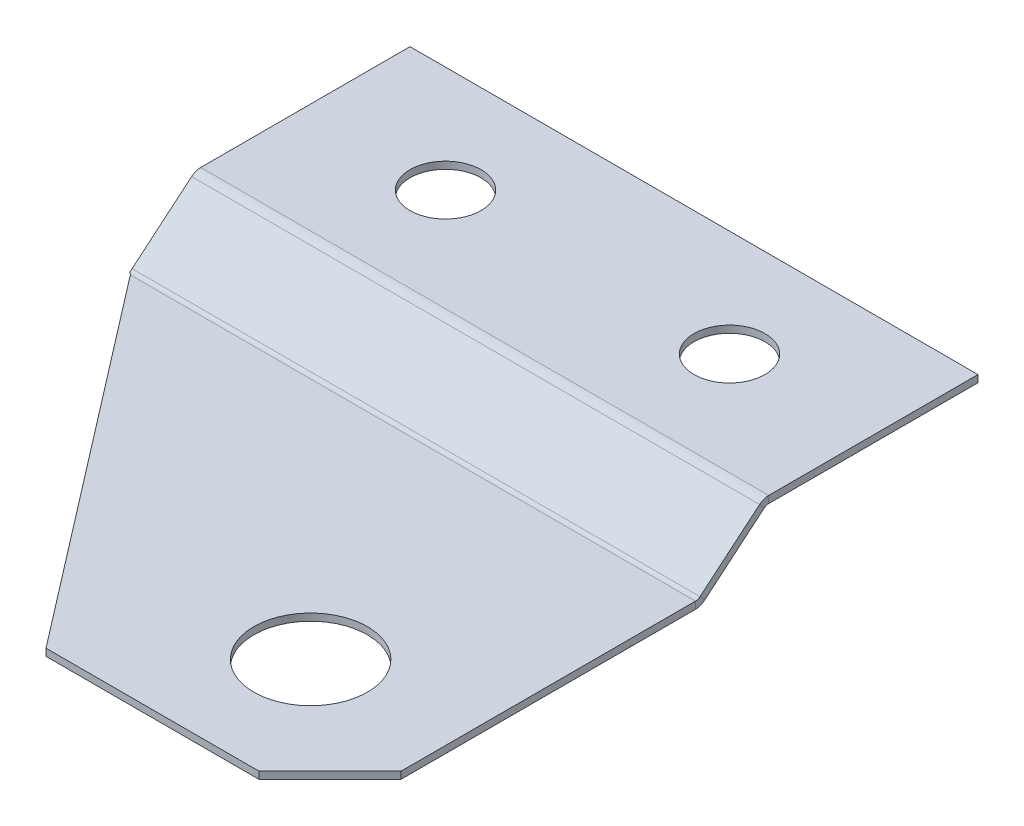
ISO-10303-21;
HEADER;
FILE_DESCRIPTION(('STEP AP214'),'2;1');
FILE_NAME('part.step','',(''),(''),'','','');
FILE_SCHEMA(('AUTOMOTIVE_DESIGN { 1 0 10303 214 1 1 1 1 }'));
ENDSEC;
DATA;
#1=APPLICATION_CONTEXT('core data for automotive mechanical design processes');
#2=APPLICATION_PROTOCOL_DEFINITION('international standard','automotive_design',2000,#1);
#3=PRODUCT_CONTEXT('',#1,'mechanical');
#4=PRODUCT('Part','Part','',(#3));
#5=PRODUCT_RELATED_PRODUCT_CATEGORY('part','',(#4));
#6=PRODUCT_DEFINITION_FORMATION('','',#4);
#7=PRODUCT_DEFINITION_CONTEXT('part definition',#1,'design');
#8=PRODUCT_DEFINITION('design','',#6,#7);
#9=PRODUCT_DEFINITION_SHAPE('','',#8);
#10=(LENGTH_UNIT() NAMED_UNIT(*) SI_UNIT(.MILLI.,.METRE.));
#11=(NAMED_UNIT(*) PLANE_ANGLE_UNIT() SI_UNIT($,.RADIAN.));
#12=(NAMED_UNIT(*) SI_UNIT($,.STERADIAN.) SOLID_ANGLE_UNIT());
#13=UNCERTAINTY_MEASURE_WITH_UNIT(LENGTH_MEASURE(1.E-05),#10,'distance_accuracy_value','');
#14=(GEOMETRIC_REPRESENTATION_CONTEXT(3) GLOBAL_UNCERTAINTY_ASSIGNED_CONTEXT((#13)) GLOBAL_UNIT_ASSIGNED_CONTEXT((#10,
#11,#12)) REPRESENTATION_CONTEXT('',''));
#15=CARTESIAN_POINT('',(0.,0.,0.));
#16=DIRECTION('',(0.,0.,1.));
#17=DIRECTION('',(1.,0.,0.));
#18=AXIS2_PLACEMENT_3D('',#15,#16,#17);
#19=CARTESIAN_POINT('',(0.,2.44384786784973,0.911844456773233));
#20=DIRECTION('',(0.,0.766044443118977,0.642787609686541));
#21=DIRECTION('',(0.,-0.642787609686541,0.766044443118977));
#22=AXIS2_PLACEMENT_3D('',#19,#20,#21);
#23=PLANE('',#22);
#24=DIRECTION('',(0.,0.64278760968654,-0.766044443118977));
#25=VECTOR('',#24,1.);
#26=CARTESIAN_POINT('',(20.,9.19311776955841,-7.13162219597603));
#27=LINE('',#26,#25);
#28=CARTESIAN_POINT('',(20.,-4.13714063115813,8.75476114328701));
#29=VERTEX_POINT('',#28);
#30=CARTESIAN_POINT('',(20.,-0.616977778440511,4.55959441704411));
#31=VERTEX_POINT('',#30);
#32=EDGE_CURVE('E375',#29,#31,#27,.T.);
#33=ORIENTED_EDGE('',*,*,#32,.F.);
#34=DIRECTION('',(-1.,0.,0.));
#35=VECTOR('',#34,1.);
#36=CARTESIAN_POINT('',(0.,-4.13714063115813,8.754761143287));
#37=LINE('',#36,#35);
#38=CARTESIAN_POINT('',(-20.,-4.13714063115813,8.75476114328701));
#39=VERTEX_POINT('',#38);
#40=EDGE_CURVE('E361',#29,#39,#37,.T.);
#41=ORIENTED_EDGE('',*,*,#40,.T.);
#42=DIRECTION('',(0.,-0.64278760968654,0.766044443118977));
#43=VECTOR('',#42,1.);
#44=CARTESIAN_POINT('',(-20.,9.19311776955841,-7.13162219597603));
#45=LINE('',#44,#43);
#46=CARTESIAN_POINT('',(-20.,-0.61697777844051,4.55959441704412));
#47=VERTEX_POINT('',#46);
#48=EDGE_CURVE('E357',#47,#39,#45,.T.);
#49=ORIENTED_EDGE('',*,*,#48,.F.);
#50=DIRECTION('',(-1.,0.,0.));
#51=VECTOR('',#50,1.);
#52=CARTESIAN_POINT('',(0.,-0.616977778440513,4.55959441704412));
#53=LINE('',#52,#51);
#54=EDGE_CURVE('E352',#31,#47,#53,.T.);
#55=ORIENTED_EDGE('',*,*,#54,.F.);
#56=EDGE_LOOP('',(#33,#41,#49,#55));
#57=FACE_BOUND('',#56,.T.);
#58=ADVANCED_FACE('F56',(#57),#23,.F.);
#59=CARTESIAN_POINT('',(20.,9.19311776955841,-7.13162219597603));
#60=DIRECTION('',(1.,0.,0.));
#61=DIRECTION('',(0.,0.642787609686541,-0.766044443118977));
#62=AXIS2_PLACEMENT_3D('',#59,#60,#61);
#63=PLANE('',#62);
#64=DIRECTION('',(0.,0.766044443118977,0.64278760968654));
#65=VECTOR('',#64,1.);
#66=CARTESIAN_POINT('',(20.,-4.13714063115813,8.75476114328701));
#67=LINE('',#66,#65);
#68=CARTESIAN_POINT('',(20.,-3.75411840959864,9.07615494813028));
#69=VERTEX_POINT('',#68);
#70=EDGE_CURVE('E366',#29,#69,#67,.T.);
#71=ORIENTED_EDGE('',*,*,#70,.F.);
#72=ORIENTED_EDGE('',*,*,#32,.T.);
#73=DIRECTION('',(0.,0.766044443118977,0.642787609686541));
#74=VECTOR('',#73,1.);
#75=CARTESIAN_POINT('',(20.,-0.616977778440512,4.55959441704412));
#76=LINE('',#75,#74);
#77=CARTESIAN_POINT('',(20.,-0.233955556881022,4.88098822188738));
#78=VERTEX_POINT('',#77);
#79=EDGE_CURVE('E363',#31,#78,#76,.T.);
#80=ORIENTED_EDGE('',*,*,#79,.T.);
#81=DIRECTION('',(0.,0.64278760968654,-0.766044443118977));
#82=VECTOR('',#81,1.);
#83=CARTESIAN_POINT('',(20.,9.5761399911179,-6.81022839113276));
#84=LINE('',#83,#82);
#85=EDGE_CURVE('E86',#69,#78,#84,.T.);
#86=ORIENTED_EDGE('',*,*,#85,.F.);
#87=EDGE_LOOP('',(#71,#72,#80,#86));
#88=FACE_BOUND('',#87,.T.);
#89=ADVANCED_FACE('F425',(#88),#63,.T.);
#90=CARTESIAN_POINT('',(-20.,9.19311776955841,-7.13162219597603));
#91=DIRECTION('',(-1.,0.,0.));
#92=DIRECTION('',(0.,-0.642787609686541,0.766044443118977));
#93=AXIS2_PLACEMENT_3D('',#90,#91,#92);
#94=PLANE('',#93);
#95=DIRECTION('',(0.,-0.766044443118977,-0.64278760968654));
#96=VECTOR('',#95,1.);
#97=CARTESIAN_POINT('',(-20.,-4.13714063115812,8.754761143287));
#98=LINE('',#97,#96);
#99=CARTESIAN_POINT('',(-20.,-3.75411840959864,9.07615494813028));
#100=VERTEX_POINT('',#99);
#101=EDGE_CURVE('E12',#100,#39,#98,.T.);
#102=ORIENTED_EDGE('',*,*,#101,.F.);
#103=DIRECTION('',(0.,-0.64278760968654,0.766044443118977));
#104=VECTOR('',#103,1.);
#105=CARTESIAN_POINT('',(-20.,9.5761399911179,-6.81022839113276));
#106=LINE('',#105,#104);
#107=CARTESIAN_POINT('',(-20.,-0.233955556881022,4.88098822188738));
#108=VERTEX_POINT('',#107);
#109=EDGE_CURVE('E76',#108,#100,#106,.T.);
#110=ORIENTED_EDGE('',*,*,#109,.F.);
#111=DIRECTION('',(0.,-0.766044443118977,-0.642787609686541));
#112=VECTOR('',#111,1.);
#113=CARTESIAN_POINT('',(-20.,-0.616977778440512,4.55959441704412));
#114=LINE('',#113,#112);
#115=EDGE_CURVE('E358',#108,#47,#114,.T.);
#116=ORIENTED_EDGE('',*,*,#115,.T.);
#117=ORIENTED_EDGE('',*,*,#48,.T.);
#118=EDGE_LOOP('',(#102,#110,#116,#117));
#119=FACE_BOUND('',#118,.T.);
#120=ADVANCED_FACE('F431',(#119),#94,.T.);
#121=CARTESIAN_POINT('',(0.,2.82687008940922,1.2332382616165));
#122=DIRECTION('',(0.,0.766044443118977,0.642787609686541));
#123=DIRECTION('',(0.,-0.642787609686541,0.766044443118977));
#124=AXIS2_PLACEMENT_3D('',#121,#122,#123);
#125=PLANE('',#124);
#126=DIRECTION('',(-1.,0.,0.));
#127=VECTOR('',#126,1.);
#128=CARTESIAN_POINT('',(0.,-3.75411840959864,9.07615494813028));
#129=LINE('',#128,#127);
#130=EDGE_CURVE('E67',#69,#100,#129,.T.);
#131=ORIENTED_EDGE('',*,*,#130,.F.);
#132=ORIENTED_EDGE('',*,*,#85,.T.);
#133=DIRECTION('',(-1.,0.,0.));
#134=VECTOR('',#133,1.);
#135=CARTESIAN_POINT('',(0.,-0.233955556881024,4.88098822188739));
#136=LINE('',#135,#134);
#137=EDGE_CURVE('E360',#78,#108,#136,.T.);
#138=ORIENTED_EDGE('',*,*,#137,.T.);
#139=ORIENTED_EDGE('',*,*,#109,.T.);
#140=EDGE_LOOP('',(#131,#132,#138,#139));
#141=FACE_BOUND('',#140,.T.);
#142=ADVANCED_FACE('F63',(#141),#125,.T.);
#143=CARTESIAN_POINT('',(-20.,-0.5,-10.5));
#144=DIRECTION('',(0.,0.,-1.));
#145=DIRECTION('',(-1.,0.,0.));
#146=AXIS2_PLACEMENT_3D('',#143,#144,#145);
#147=PLANE('',#146);
#148=DIRECTION('',(-1.,0.,0.));
#149=VECTOR('',#148,1.);
#150=CARTESIAN_POINT('',(-20.,0.,-10.5));
#151=LINE('',#150,#149);
#152=CARTESIAN_POINT('',(20.,0.,-10.5));
#153=VERTEX_POINT('',#152);
#154=CARTESIAN_POINT('',(-20.,0.,-10.5));
#155=VERTEX_POINT('',#154);
#156=EDGE_CURVE('E327',#153,#155,#151,.T.);
#157=ORIENTED_EDGE('',*,*,#156,.F.);
#158=DIRECTION('',(0.,1.,0.));
#159=VECTOR('',#158,1.);
#160=CARTESIAN_POINT('',(20.,-0.5,-10.5));
#161=LINE('',#160,#159);
#162=CARTESIAN_POINT('',(20.,-0.5,-10.5));
#163=VERTEX_POINT('',#162);
#164=EDGE_CURVE('E321',#163,#153,#161,.T.);
#165=ORIENTED_EDGE('',*,*,#164,.F.);
#166=DIRECTION('',(-1.,0.,0.));
#167=VECTOR('',#166,1.);
#168=CARTESIAN_POINT('',(-20.,-0.5,-10.5));
#169=LINE('',#168,#167);
#170=CARTESIAN_POINT('',(-20.,-0.5,-10.5));
#171=VERTEX_POINT('',#170);
#172=EDGE_CURVE('E345',#163,#171,#169,.T.);
#173=ORIENTED_EDGE('',*,*,#172,.T.);
#174=DIRECTION('',(0.,1.,0.));
#175=VECTOR('',#174,1.);
#176=CARTESIAN_POINT('',(-20.,-0.5,-10.5));
#177=LINE('',#176,#175);
#178=EDGE_CURVE('E338',#171,#155,#177,.T.);
#179=ORIENTED_EDGE('',*,*,#178,.T.);
#180=EDGE_LOOP('',(#157,#165,#173,#179));
#181=FACE_BOUND('',#180,.T.);
#182=ADVANCED_FACE('F455',(#181),#147,.T.);
#183=CARTESIAN_POINT('',(0.,-0.5,0.));
#184=DIRECTION('',(0.,1.,0.));
#185=DIRECTION('',(0.,0.,1.));
#186=AXIS2_PLACEMENT_3D('',#183,#184,#185);
#187=PLANE('',#186);
#188=CARTESIAN_POINT('',(-10.,-0.5,-3.));
#189=DIRECTION('',(0.,1.,0.));
#190=DIRECTION('',(0.,0.,1.));
#191=AXIS2_PLACEMENT_3D('',#188,#189,#190);
#192=CIRCLE('',#191,2.5);
#193=CARTESIAN_POINT('',(-10.,-0.5,-0.500000000000002));
#194=VERTEX_POINT('',#193);
#195=EDGE_CURVE('E195',#194,#194,#192,.T.);
#196=ORIENTED_EDGE('',*,*,#195,.T.);
#197=EDGE_LOOP('',(#196));
#198=FACE_BOUND('',#197,.T.);
#199=CARTESIAN_POINT('',(10.,-0.5,-3.));
#200=DIRECTION('',(0.,1.,0.));
#201=DIRECTION('',(0.,0.,1.));
#202=AXIS2_PLACEMENT_3D('',#199,#200,#201);
#203=CIRCLE('',#202,2.5);
#204=CARTESIAN_POINT('',(10.,-0.5,-0.500000000000002));
#205=VERTEX_POINT('',#204);
#206=EDGE_CURVE('E650',#205,#205,#203,.T.);
#207=ORIENTED_EDGE('',*,*,#206,.T.);
#208=EDGE_LOOP('',(#207));
#209=FACE_BOUND('',#208,.T.);
#210=DIRECTION('',(0.,0.,-1.));
#211=VECTOR('',#210,1.);
#212=CARTESIAN_POINT('',(20.,-0.5,-10.5));
#213=LINE('',#212,#211);
#214=CARTESIAN_POINT('',(20.,-0.5,4.23820061220084));
#215=VERTEX_POINT('',#214);
#216=EDGE_CURVE('E329',#215,#163,#213,.T.);
#217=ORIENTED_EDGE('',*,*,#216,.F.);
#218=DIRECTION('',(-1.,0.,0.));
#219=VECTOR('',#218,1.);
#220=CARTESIAN_POINT('',(0.,-0.5,4.23820061220085));
#221=LINE('',#220,#219);
#222=CARTESIAN_POINT('',(-20.,-0.5,4.23820061220084));
#223=VERTEX_POINT('',#222);
#224=EDGE_CURVE('E340',#215,#223,#221,.T.);
#225=ORIENTED_EDGE('',*,*,#224,.T.);
#226=DIRECTION('',(0.,0.,1.));
#227=VECTOR('',#226,1.);
#228=CARTESIAN_POINT('',(-20.,-0.5,-10.5));
#229=LINE('',#228,#227);
#230=EDGE_CURVE('E334',#171,#223,#229,.T.);
#231=ORIENTED_EDGE('',*,*,#230,.F.);
#232=ORIENTED_EDGE('',*,*,#172,.F.);
#233=EDGE_LOOP('',(#217,#225,#231,#232));
#234=FACE_BOUND('',#233,.T.);
#235=ADVANCED_FACE('F449',(#198,#209,#234),#187,.F.);
#236=CARTESIAN_POINT('',(-20.,-0.5,-10.5));
#237=DIRECTION('',(-1.,0.,0.));
#238=DIRECTION('',(0.,0.,1.));
#239=AXIS2_PLACEMENT_3D('',#236,#237,#238);
#240=PLANE('',#239);
#241=DIRECTION('',(0.,-1.,0.));
#242=VECTOR('',#241,1.);
#243=CARTESIAN_POINT('',(-20.,-0.499999999999999,4.23820061220085));
#244=LINE('',#243,#242);
#245=CARTESIAN_POINT('',(-20.,0.,4.23820061220084));
#246=VERTEX_POINT('',#245);
#247=EDGE_CURVE('E342',#246,#223,#244,.T.);
#248=ORIENTED_EDGE('',*,*,#247,.F.);
#249=DIRECTION('',(0.,0.,1.));
#250=VECTOR('',#249,1.);
#251=CARTESIAN_POINT('',(-20.,0.,-10.5));
#252=LINE('',#251,#250);
#253=EDGE_CURVE('E330',#155,#246,#252,.T.);
#254=ORIENTED_EDGE('',*,*,#253,.F.);
#255=ORIENTED_EDGE('',*,*,#178,.F.);
#256=ORIENTED_EDGE('',*,*,#230,.T.);
#257=EDGE_LOOP('',(#248,#254,#255,#256));
#258=FACE_BOUND('',#257,.T.);
#259=ADVANCED_FACE('F443',(#258),#240,.T.);
#260=CARTESIAN_POINT('',(0.,0.,0.));
#261=DIRECTION('',(0.,1.,0.));
#262=DIRECTION('',(0.,0.,1.));
#263=AXIS2_PLACEMENT_3D('',#260,#261,#262);
#264=PLANE('',#263);
#265=CARTESIAN_POINT('',(-10.,0.,-3.));
#266=DIRECTION('',(0.,1.,0.));
#267=DIRECTION('',(0.,0.,1.));
#268=AXIS2_PLACEMENT_3D('',#265,#266,#267);
#269=CIRCLE('',#268,2.5);
#270=CARTESIAN_POINT('',(-10.,0.,-0.500000000000002));
#271=VERTEX_POINT('',#270);
#272=EDGE_CURVE('E651',#271,#271,#269,.T.);
#273=ORIENTED_EDGE('',*,*,#272,.F.);
#274=EDGE_LOOP('',(#273));
#275=FACE_BOUND('',#274,.T.);
#276=CARTESIAN_POINT('',(10.,0.,-3.));
#277=DIRECTION('',(0.,1.,0.));
#278=DIRECTION('',(0.,0.,1.));
#279=AXIS2_PLACEMENT_3D('',#276,#277,#278);
#280=CIRCLE('',#279,2.5);
#281=CARTESIAN_POINT('',(10.,0.,-0.500000000000002));
#282=VERTEX_POINT('',#281);
#283=EDGE_CURVE('E652',#282,#282,#280,.T.);
#284=ORIENTED_EDGE('',*,*,#283,.F.);
#285=EDGE_LOOP('',(#284));
#286=FACE_BOUND('',#285,.T.);
#287=DIRECTION('',(-1.,0.,0.));
#288=VECTOR('',#287,1.);
#289=CARTESIAN_POINT('',(0.,0.,4.23820061220085));
#290=LINE('',#289,#288);
#291=CARTESIAN_POINT('',(20.,0.,4.23820061220084));
#292=VERTEX_POINT('',#291);
#293=EDGE_CURVE('E348',#292,#246,#290,.T.);
#294=ORIENTED_EDGE('',*,*,#293,.F.);
#295=DIRECTION('',(0.,0.,-1.));
#296=VECTOR('',#295,1.);
#297=CARTESIAN_POINT('',(20.,0.,-10.5));
#298=LINE('',#297,#296);
#299=EDGE_CURVE('E333',#292,#153,#298,.T.);
#300=ORIENTED_EDGE('',*,*,#299,.T.);
#301=ORIENTED_EDGE('',*,*,#156,.T.);
#302=ORIENTED_EDGE('',*,*,#253,.T.);
#303=EDGE_LOOP('',(#294,#300,#301,#302));
#304=FACE_BOUND('',#303,.T.);
#305=ADVANCED_FACE('F439',(#275,#286,#304),#264,.T.);
#306=CARTESIAN_POINT('',(20.,-0.5,-10.5));
#307=DIRECTION('',(1.,0.,0.));
#308=DIRECTION('',(0.,0.,-1.));
#309=AXIS2_PLACEMENT_3D('',#306,#307,#308);
#310=PLANE('',#309);
#311=DIRECTION('',(0.,1.,0.));
#312=VECTOR('',#311,1.);
#313=CARTESIAN_POINT('',(20.,-0.499999999999999,4.23820061220085));
#314=LINE('',#313,#312);
#315=EDGE_CURVE('E320',#215,#292,#314,.T.);
#316=ORIENTED_EDGE('',*,*,#315,.F.);
#317=ORIENTED_EDGE('',*,*,#216,.T.);
#318=ORIENTED_EDGE('',*,*,#164,.T.);
#319=ORIENTED_EDGE('',*,*,#299,.F.);
#320=EDGE_LOOP('',(#316,#317,#318,#319));
#321=FACE_BOUND('',#320,.T.);
#322=ADVANCED_FACE('F436',(#321),#310,.T.);
#323=CARTESIAN_POINT('',(20.,-1.,4.23820061220085));
#324=DIRECTION('',(-1.,0.,0.));
#325=DIRECTION('',(0.,0.,1.));
#326=AXIS2_PLACEMENT_3D('',#323,#324,#325);
#327=PLANE('',#326);
#328=ORIENTED_EDGE('',*,*,#315,.T.);
#329=CARTESIAN_POINT('',(20.,-1.,4.23820061220085));
#330=DIRECTION('',(-1.,0.,0.));
#331=DIRECTION('',(0.,0.,1.));
#332=AXIS2_PLACEMENT_3D('',#329,#330,#331);
#333=CIRCLE('',#332,1.);
#334=EDGE_CURVE('E318',#292,#78,#333,.F.);
#335=ORIENTED_EDGE('',*,*,#334,.T.);
#336=ORIENTED_EDGE('',*,*,#79,.F.);
#337=CARTESIAN_POINT('',(20.,-1.,4.23820061220085));
#338=DIRECTION('',(1.,0.,0.));
#339=DIRECTION('',(0.,0.,1.));
#340=AXIS2_PLACEMENT_3D('',#337,#338,#339);
#341=CIRCLE('',#340,0.5);
#342=EDGE_CURVE('E304',#215,#31,#341,.T.);
#343=ORIENTED_EDGE('',*,*,#342,.F.);
#344=EDGE_LOOP('',(#328,#335,#336,#343));
#345=FACE_BOUND('',#344,.T.);
#346=ADVANCED_FACE('F437',(#345),#327,.F.);
#347=CARTESIAN_POINT('',(-20.,-1.,4.23820061220085));
#348=DIRECTION('',(1.,0.,0.));
#349=DIRECTION('',(0.,0.,-1.));
#350=AXIS2_PLACEMENT_3D('',#347,#348,#349);
#351=PLANE('',#350);
#352=ORIENTED_EDGE('',*,*,#115,.F.);
#353=CARTESIAN_POINT('',(-20.,-1.,4.23820061220085));
#354=DIRECTION('',(-1.,0.,0.));
#355=DIRECTION('',(0.,0.,1.));
#356=AXIS2_PLACEMENT_3D('',#353,#354,#355);
#357=CIRCLE('',#356,1.);
#358=EDGE_CURVE('E313',#108,#246,#357,.T.);
#359=ORIENTED_EDGE('',*,*,#358,.T.);
#360=ORIENTED_EDGE('',*,*,#247,.T.);
#361=CARTESIAN_POINT('',(-20.,-1.,4.23820061220085));
#362=DIRECTION('',(-1.,0.,0.));
#363=DIRECTION('',(0.,0.,-1.));
#364=AXIS2_PLACEMENT_3D('',#361,#362,#363);
#365=CIRCLE('',#364,0.5);
#366=EDGE_CURVE('E312',#47,#223,#365,.T.);
#367=ORIENTED_EDGE('',*,*,#366,.F.);
#368=EDGE_LOOP('',(#352,#359,#360,#367));
#369=FACE_BOUND('',#368,.T.);
#370=ADVANCED_FACE('F458',(#369),#351,.F.);
#371=CARTESIAN_POINT('',(40.0065514094605,-1.,4.23820061220085));
#372=DIRECTION('',(-1.,0.,0.));
#373=DIRECTION('',(0.,0.,1.));
#374=AXIS2_PLACEMENT_3D('',#371,#372,#373);
#375=CYLINDRICAL_SURFACE('',#374,0.5);
#376=ORIENTED_EDGE('',*,*,#366,.T.);
#377=ORIENTED_EDGE('',*,*,#224,.F.);
#378=ORIENTED_EDGE('',*,*,#342,.T.);
#379=ORIENTED_EDGE('',*,*,#54,.T.);
#380=EDGE_LOOP('',(#376,#377,#378,#379));
#381=FACE_BOUND('',#380,.T.);
#382=ADVANCED_FACE('F463',(#381),#375,.F.);
#383=CARTESIAN_POINT('',(40.0065514094605,-1.,4.23820061220085));
#384=DIRECTION('',(-1.,0.,0.));
#385=DIRECTION('',(0.,0.,1.));
#386=AXIS2_PLACEMENT_3D('',#383,#384,#385);
#387=CYLINDRICAL_SURFACE('',#386,1.);
#388=ORIENTED_EDGE('',*,*,#358,.F.);
#389=ORIENTED_EDGE('',*,*,#137,.F.);
#390=ORIENTED_EDGE('',*,*,#334,.F.);
#391=ORIENTED_EDGE('',*,*,#293,.T.);
#392=EDGE_LOOP('',(#388,#389,#390,#391));
#393=FACE_BOUND('',#392,.T.);
#394=ADVANCED_FACE('F464',(#393),#387,.T.);
#395=CARTESIAN_POINT('',(20.,-3.37109618803915,9.39754875297355));
#396=DIRECTION('',(1.,0.,0.));
#397=DIRECTION('',(0.,0.,-1.));
#398=AXIS2_PLACEMENT_3D('',#395,#396,#397);
#399=PLANE('',#398);
#400=ORIENTED_EDGE('',*,*,#70,.T.);
#401=CARTESIAN_POINT('',(20.,-3.37109618803915,9.39754875297355));
#402=DIRECTION('',(-1.,0.,0.));
#403=DIRECTION('',(0.,0.,1.));
#404=AXIS2_PLACEMENT_3D('',#401,#402,#403);
#405=CIRCLE('',#404,0.5);
#406=CARTESIAN_POINT('',(20.,-3.87109618803915,9.39754875297355));
#407=VERTEX_POINT('',#406);
#408=EDGE_CURVE('E185',#69,#407,#405,.T.);
#409=ORIENTED_EDGE('',*,*,#408,.T.);
#410=DIRECTION('',(0.,1.,0.));
#411=VECTOR('',#410,1.);
#412=CARTESIAN_POINT('',(20.,-4.37109618803915,9.39754875297355));
#413=LINE('',#412,#411);
#414=CARTESIAN_POINT('',(20.,-4.37109618803915,9.39754875297355));
#415=VERTEX_POINT('',#414);
#416=EDGE_CURVE('E394',#415,#407,#413,.T.);
#417=ORIENTED_EDGE('',*,*,#416,.F.);
#418=CARTESIAN_POINT('',(20.,-3.37109618803915,9.39754875297355));
#419=DIRECTION('',(-1.,0.,0.));
#420=DIRECTION('',(0.,0.,-1.));
#421=AXIS2_PLACEMENT_3D('',#418,#419,#420);
#422=CIRCLE('',#421,1.);
#423=EDGE_CURVE('E199',#29,#415,#422,.T.);
#424=ORIENTED_EDGE('',*,*,#423,.F.);
#425=EDGE_LOOP('',(#400,#409,#417,#424));
#426=FACE_BOUND('',#425,.T.);
#427=ADVANCED_FACE('F266',(#426),#399,.T.);
#428=CARTESIAN_POINT('',(-19.7986158555391,-4.37109618803915,9.39754875297352));
#429=CARTESIAN_POINT('',(-19.865763977686,-4.37109618803915,9.2811586745856));
#430=CARTESIAN_POINT('',(-19.9328518778531,-4.35059656011698,9.1648995074417));
#431=CARTESIAN_POINT('',(-20.,-4.31078880882506,9.05552860964787));
#432=CARTESIAN_POINT('',(-19.7986158555391,-3.87109618803915,9.39754875297353));
#433=CARTESIAN_POINT('',(-19.8657560024041,-3.87109618803915,9.33936062569053));
#434=CARTESIAN_POINT('',(-19.932859853135,-3.86084401006529,9.2812176351359));
#435=CARTESIAN_POINT('',(-20.,-3.8409424984321,9.22653868131071));
#436=B_SPLINE_SURFACE_WITH_KNOTS('',1,3,((#428,#429,#430,#431),(#432,#433,#434,#435)),
.UNSPECIFIED.,.F.,.F.,.F.,(2,2),(4,4),(0.,1.),(0.,1.),.UNSPECIFIED.);
#437=CARTESIAN_POINT('',(-19.7986158555391,-4.37109618803915,9.39754875297352));
#438=CARTESIAN_POINT('',(-19.7986158555391,-3.87109618803915,9.39754875297353));
#439=B_SPLINE_CURVE_WITH_KNOTS('',1,(#437,#438),.UNSPECIFIED.,.F.,.F.,(2,2),(0.,1.),.UNSPECIFIED.);
#440=CARTESIAN_POINT('',(-19.7986158555391,-3.87109618803914,9.39754875297354));
#441=VERTEX_POINT('',#440);
#442=CARTESIAN_POINT('',(-19.7986158555391,-4.37109618803915,9.39754875297352));
#443=VERTEX_POINT('',#442);
#444=EDGE_CURVE('E171',#441,#443,#439,.F.);
#445=CARTESIAN_POINT('',(-19.7986158555391,-3.87109618803915,9.39754875297353));
#446=CARTESIAN_POINT('',(-19.8657560024041,-3.87109618803915,9.33936062569053));
#447=CARTESIAN_POINT('',(-19.932859853135,-3.86084401006529,9.2812176351359));
#448=CARTESIAN_POINT('',(-20.,-3.8409424984321,9.22653868131071));
#449=B_SPLINE_CURVE_WITH_KNOTS('',3,(#445,#446,#447,#448),.UNSPECIFIED.,.F.,.F.,(4,4),(0.,1.),.UNSPECIFIED.);
#450=CARTESIAN_POINT('',(-20.,-3.8409424984321,9.22653868131071));
#451=VERTEX_POINT('',#450);
#452=EDGE_CURVE('E203',#441,#451,#449,.T.);
#453=CARTESIAN_POINT('',(-20.,-3.8409424984321,9.22653868131071));
#454=CARTESIAN_POINT('',(-20.,-4.31078880882506,9.05552860964787));
#455=B_SPLINE_CURVE_WITH_KNOTS('',1,(#453,#454),.UNSPECIFIED.,.F.,.F.,(2,2),(0.,1.),.UNSPECIFIED.);
#456=CARTESIAN_POINT('',(-20.,-4.31078880882506,9.05552860964787));
#457=VERTEX_POINT('',#456);
#458=EDGE_CURVE('E292',#451,#457,#455,.T.);
#459=CARTESIAN_POINT('',(-20.,-4.31078880882506,9.05552860964787));
#460=CARTESIAN_POINT('',(-19.9328518778531,-4.35059656011698,9.1648995074417));
#461=CARTESIAN_POINT('',(-19.865763977686,-4.37109618803915,9.2811586745856));
#462=CARTESIAN_POINT('',(-19.7986158555391,-4.37109618803915,9.39754875297352));
#463=B_SPLINE_CURVE_WITH_KNOTS('',3,(#459,#460,#461,#462),.UNSPECIFIED.,.F.,.F.,(4,4),(0.,1.),.UNSPECIFIED.);
#464=EDGE_CURVE('E198',#443,#457,#463,.F.);
#465=ORIENTED_EDGE('',*,*,#444,.F.);
#466=ORIENTED_EDGE('',*,*,#452,.T.);
#467=ORIENTED_EDGE('',*,*,#458,.T.);
#468=ORIENTED_EDGE('',*,*,#464,.F.);
#469=EDGE_LOOP('',(#465,#466,#467,#468));
#470=FACE_BOUND('',#469,.T.);
#471=ADVANCED_FACE('F253',(#470),#436,.T.);
#472=CARTESIAN_POINT('',(-20.,-3.37109618803915,9.39754875297354));
#473=DIRECTION('',(-1.,-1.27802273608187E-13,1.52308818714266E-13));
#474=DIRECTION('',(1.52308818714266E-13,0.,1.));
#475=AXIS2_PLACEMENT_3D('',#472,#473,#474);
#476=PLANE('',#475);
#477=ORIENTED_EDGE('',*,*,#458,.F.);
#478=CARTESIAN_POINT('',(-20.,-3.37109618803915,9.39754875297354));
#479=DIRECTION('',(-1.,0.,0.));
#480=DIRECTION('',(0.,0.,1.));
#481=AXIS2_PLACEMENT_3D('',#478,#479,#480);
#482=CIRCLE('',#481,0.5);
#483=EDGE_CURVE('E197',#451,#100,#482,.F.);
#484=ORIENTED_EDGE('',*,*,#483,.T.);
#485=ORIENTED_EDGE('',*,*,#101,.T.);
#486=CARTESIAN_POINT('',(-20.,-3.37109618803915,9.39754875297354));
#487=DIRECTION('',(1.,1.27802273608187E-13,-1.52308818714266E-13));
#488=DIRECTION('',(1.52308818714266E-13,0.,1.));
#489=AXIS2_PLACEMENT_3D('',#486,#487,#488);
#490=CIRCLE('',#489,1.);
#491=EDGE_CURVE('E215',#457,#39,#490,.T.);
#492=ORIENTED_EDGE('',*,*,#491,.F.);
#493=EDGE_LOOP('',(#477,#484,#485,#492));
#494=FACE_BOUND('',#493,.T.);
#495=ADVANCED_FACE('F224',(#494),#476,.T.);
#496=CARTESIAN_POINT('',(40.0129953866426,-3.37109618803916,9.39754875297355));
#497=DIRECTION('',(-1.,0.,0.));
#498=DIRECTION('',(0.,0.,1.));
#499=AXIS2_PLACEMENT_3D('',#496,#497,#498);
#500=CYLINDRICAL_SURFACE('',#499,1.);
#501=ORIENTED_EDGE('',*,*,#491,.T.);
#502=ORIENTED_EDGE('',*,*,#40,.F.);
#503=ORIENTED_EDGE('',*,*,#423,.T.);
#504=DIRECTION('',(-1.,0.,0.));
#505=VECTOR('',#504,1.);
#506=CARTESIAN_POINT('',(0.,-4.37109618803914,9.39754875297355));
#507=LINE('',#506,#505);
#508=EDGE_CURVE('E186',#415,#443,#507,.T.);
#509=ORIENTED_EDGE('',*,*,#508,.T.);
#510=ORIENTED_EDGE('',*,*,#464,.T.);
#511=EDGE_LOOP('',(#501,#502,#503,#509,#510));
#512=FACE_BOUND('',#511,.T.);
#513=ADVANCED_FACE('F212',(#512),#500,.T.);
#514=CARTESIAN_POINT('',(40.0129953866426,-3.37109618803916,9.39754875297355));
#515=DIRECTION('',(-1.,0.,0.));
#516=DIRECTION('',(0.,0.,1.));
#517=AXIS2_PLACEMENT_3D('',#514,#515,#516);
#518=CYLINDRICAL_SURFACE('',#517,0.5);
#519=ORIENTED_EDGE('',*,*,#483,.F.);
#520=ORIENTED_EDGE('',*,*,#452,.F.);
#521=DIRECTION('',(-1.,0.,0.));
#522=VECTOR('',#521,1.);
#523=CARTESIAN_POINT('',(0.,-3.87109618803914,9.39754875297354));
#524=LINE('',#523,#522);
#525=EDGE_CURVE('E385',#407,#441,#524,.T.);
#526=ORIENTED_EDGE('',*,*,#525,.F.);
#527=ORIENTED_EDGE('',*,*,#408,.F.);
#528=ORIENTED_EDGE('',*,*,#130,.T.);
#529=EDGE_LOOP('',(#519,#520,#526,#527,#528));
#530=FACE_BOUND('',#529,.T.);
#531=ADVANCED_FACE('F223',(#530),#518,.F.);
#532=CARTESIAN_POINT('',(15.,-4.37109618803915,35.1357493651744));
#533=DIRECTION('',(0.,0.,1.));
#534=DIRECTION('',(1.,0.,0.));
#535=AXIS2_PLACEMENT_3D('',#532,#533,#534);
#536=PLANE('',#535);
#537=DIRECTION('',(1.,0.,0.));
#538=VECTOR('',#537,1.);
#539=CARTESIAN_POINT('',(15.,-3.87109618803915,35.1357493651744));
#540=LINE('',#539,#538);
#541=CARTESIAN_POINT('',(0.,-3.87109618803914,35.1357493651744));
#542=VERTEX_POINT('',#541);
#543=CARTESIAN_POINT('',(15.,-3.87109618803915,35.1357493651744));
#544=VERTEX_POINT('',#543);
#545=EDGE_CURVE('E181',#542,#544,#540,.T.);
#546=ORIENTED_EDGE('',*,*,#545,.F.);
#547=DIRECTION('',(0.,1.,0.));
#548=VECTOR('',#547,1.);
#549=CARTESIAN_POINT('',(0.,-4.37109618803914,35.1357493651744));
#550=LINE('',#549,#548);
#551=CARTESIAN_POINT('',(0.,-4.37109618803914,35.1357493651744));
#552=VERTEX_POINT('',#551);
#553=EDGE_CURVE('E166',#552,#542,#550,.T.);
#554=ORIENTED_EDGE('',*,*,#553,.F.);
#555=DIRECTION('',(1.,0.,0.));
#556=VECTOR('',#555,1.);
#557=CARTESIAN_POINT('',(15.,-4.37109618803915,35.1357493651744));
#558=LINE('',#557,#556);
#559=CARTESIAN_POINT('',(15.,-4.37109618803915,35.1357493651744));
#560=VERTEX_POINT('',#559);
#561=EDGE_CURVE('E177',#552,#560,#558,.T.);
#562=ORIENTED_EDGE('',*,*,#561,.T.);
#563=DIRECTION('',(0.,1.,0.));
#564=VECTOR('',#563,1.);
#565=CARTESIAN_POINT('',(15.,-4.37109618803915,35.1357493651744));
#566=LINE('',#565,#564);
#567=EDGE_CURVE('E189',#560,#544,#566,.T.);
#568=ORIENTED_EDGE('',*,*,#567,.T.);
#569=EDGE_LOOP('',(#546,#554,#562,#568));
#570=FACE_BOUND('',#569,.T.);
#571=ADVANCED_FACE('F178',(#570),#536,.T.);
#572=CARTESIAN_POINT('',(20.,-4.37109618803915,30.1357493651744));
#573=DIRECTION('',(0.707106781186547,0.,0.707106781186548));
#574=DIRECTION('',(0.707106781186548,0.,-0.707106781186548));
#575=AXIS2_PLACEMENT_3D('',#572,#573,#574);
#576=PLANE('',#575);
#577=DIRECTION('',(0.707106781186548,0.,-0.707106781186548));
#578=VECTOR('',#577,1.);
#579=CARTESIAN_POINT('',(20.,-3.87109618803915,30.1357493651744));
#580=LINE('',#579,#578);
#581=CARTESIAN_POINT('',(20.,-3.87109618803915,30.1357493651744));
#582=VERTEX_POINT('',#581);
#583=EDGE_CURVE('E406',#544,#582,#580,.T.);
#584=ORIENTED_EDGE('',*,*,#583,.F.);
#585=ORIENTED_EDGE('',*,*,#567,.F.);
#586=DIRECTION('',(0.707106781186548,0.,-0.707106781186548));
#587=VECTOR('',#586,1.);
#588=CARTESIAN_POINT('',(20.,-4.37109618803915,30.1357493651744));
#589=LINE('',#588,#587);
#590=CARTESIAN_POINT('',(20.,-4.37109618803915,30.1357493651744));
#591=VERTEX_POINT('',#590);
#592=EDGE_CURVE('E190',#560,#591,#589,.T.);
#593=ORIENTED_EDGE('',*,*,#592,.T.);
#594=DIRECTION('',(0.,1.,0.));
#595=VECTOR('',#594,1.);
#596=CARTESIAN_POINT('',(20.,-4.37109618803915,30.1357493651744));
#597=LINE('',#596,#595);
#598=EDGE_CURVE('E405',#591,#582,#597,.T.);
#599=ORIENTED_EDGE('',*,*,#598,.T.);
#600=EDGE_LOOP('',(#584,#585,#593,#599));
#601=FACE_BOUND('',#600,.T.);
#602=ADVANCED_FACE('F408',(#601),#576,.T.);
#603=CARTESIAN_POINT('',(0.,-4.37109618803914,-1.36425063482561));
#604=DIRECTION('',(0.,1.,0.));
#605=DIRECTION('',(0.,0.,1.));
#606=AXIS2_PLACEMENT_3D('',#603,#604,#605);
#607=PLANE('',#606);
#608=CARTESIAN_POINT('',(10.,-4.37109618803914,26.5));
#609=DIRECTION('',(0.,1.,0.));
#610=DIRECTION('',(-1.,0.,0.));
#611=AXIS2_PLACEMENT_3D('',#608,#609,#610);
#612=CIRCLE('',#611,4.);
#613=CARTESIAN_POINT('',(6.00000000000001,-4.37109618803914,26.5));
#614=VERTEX_POINT('',#613);
#615=EDGE_CURVE('E644',#614,#614,#612,.T.);
#616=ORIENTED_EDGE('',*,*,#615,.T.);
#617=EDGE_LOOP('',(#616));
#618=FACE_BOUND('',#617,.T.);
#619=ORIENTED_EDGE('',*,*,#508,.F.);
#620=DIRECTION('',(0.,0.,-1.));
#621=VECTOR('',#620,1.);
#622=CARTESIAN_POINT('',(20.,-4.37109618803915,-11.8642506348256));
#623=LINE('',#622,#621);
#624=EDGE_CURVE('E392',#591,#415,#623,.T.);
#625=ORIENTED_EDGE('',*,*,#624,.F.);
#626=ORIENTED_EDGE('',*,*,#592,.F.);
#627=ORIENTED_EDGE('',*,*,#561,.F.);
#628=DIRECTION('',(0.609710760849692,0.,0.7926239891046));
#629=VECTOR('',#628,1.);
#630=CARTESIAN_POINT('',(0.,-4.37109618803914,35.1357493651744));
#631=LINE('',#630,#629);
#632=EDGE_CURVE('E164',#443,#552,#631,.T.);
#633=ORIENTED_EDGE('',*,*,#632,.F.);
#634=EDGE_LOOP('',(#619,#625,#626,#627,#633));
#635=FACE_BOUND('',#634,.T.);
#636=ADVANCED_FACE('F184',(#618,#635),#607,.F.);
#637=CARTESIAN_POINT('',(20.,-4.37109618803915,-11.8642506348256));
#638=DIRECTION('',(1.,0.,0.));
#639=DIRECTION('',(0.,0.,-1.));
#640=AXIS2_PLACEMENT_3D('',#637,#638,#639);
#641=PLANE('',#640);
#642=ORIENTED_EDGE('',*,*,#624,.T.);
#643=ORIENTED_EDGE('',*,*,#416,.T.);
#644=DIRECTION('',(0.,0.,-1.));
#645=VECTOR('',#644,1.);
#646=CARTESIAN_POINT('',(20.,-3.87109618803915,-11.8642506348256));
#647=LINE('',#646,#645);
#648=EDGE_CURVE('E390',#582,#407,#647,.T.);
#649=ORIENTED_EDGE('',*,*,#648,.F.);
#650=ORIENTED_EDGE('',*,*,#598,.F.);
#651=EDGE_LOOP('',(#642,#643,#649,#650));
#652=FACE_BOUND('',#651,.T.);
#653=ADVANCED_FACE('F411',(#652),#641,.T.);
#654=CARTESIAN_POINT('',(0.,-3.87109618803914,-1.36425063482561));
#655=DIRECTION('',(0.,1.,0.));
#656=DIRECTION('',(0.,0.,1.));
#657=AXIS2_PLACEMENT_3D('',#654,#655,#656);
#658=PLANE('',#657);
#659=CARTESIAN_POINT('',(10.,-3.87109618803914,26.5));
#660=DIRECTION('',(0.,1.,0.));
#661=DIRECTION('',(-1.,0.,0.));
#662=AXIS2_PLACEMENT_3D('',#659,#660,#661);
#663=CIRCLE('',#662,4.);
#664=CARTESIAN_POINT('',(6.00000000000001,-3.87109618803914,26.5));
#665=VERTEX_POINT('',#664);
#666=EDGE_CURVE('E643',#665,#665,#663,.T.);
#667=ORIENTED_EDGE('',*,*,#666,.F.);
#668=EDGE_LOOP('',(#667));
#669=FACE_BOUND('',#668,.T.);
#670=ORIENTED_EDGE('',*,*,#648,.T.);
#671=ORIENTED_EDGE('',*,*,#525,.T.);
#672=DIRECTION('',(0.609710760849692,0.,0.7926239891046));
#673=VECTOR('',#672,1.);
#674=CARTESIAN_POINT('',(0.,-3.87109618803914,35.1357493651744));
#675=LINE('',#674,#673);
#676=EDGE_CURVE('E379',#441,#542,#675,.T.);
#677=ORIENTED_EDGE('',*,*,#676,.T.);
#678=ORIENTED_EDGE('',*,*,#545,.T.);
#679=ORIENTED_EDGE('',*,*,#583,.T.);
#680=EDGE_LOOP('',(#670,#671,#677,#678,#679));
#681=FACE_BOUND('',#680,.T.);
#682=ADVANCED_FACE('F409',(#669,#681),#658,.T.);
#683=CARTESIAN_POINT('',(0.,-4.37109618803914,35.1357493651744));
#684=DIRECTION('',(-0.7926239891046,0.,0.609710760849693));
#685=DIRECTION('',(0.609710760849692,0.,0.792623989104601));
#686=AXIS2_PLACEMENT_3D('',#683,#684,#685);
#687=PLANE('',#686);
#688=ORIENTED_EDGE('',*,*,#676,.F.);
#689=ORIENTED_EDGE('',*,*,#444,.T.);
#690=ORIENTED_EDGE('',*,*,#632,.T.);
#691=ORIENTED_EDGE('',*,*,#553,.T.);
#692=EDGE_LOOP('',(#688,#689,#690,#691));
#693=FACE_BOUND('',#692,.T.);
#694=ADVANCED_FACE('F170',(#693),#687,.T.);
#695=CARTESIAN_POINT('',(10.,-0.5,-3.));
#696=DIRECTION('',(0.,1.,0.));
#697=DIRECTION('',(0.,0.,1.));
#698=AXIS2_PLACEMENT_3D('',#695,#696,#697);
#699=CYLINDRICAL_SURFACE('',#698,2.5);
#700=ORIENTED_EDGE('',*,*,#206,.F.);
#701=EDGE_LOOP('',(#700));
#702=FACE_BOUND('',#701,.T.);
#703=ORIENTED_EDGE('',*,*,#283,.T.);
#704=EDGE_LOOP('',(#703));
#705=FACE_BOUND('',#704,.T.);
#706=ADVANCED_FACE('F417',(#702,#705),#699,.F.);
#707=CARTESIAN_POINT('',(-10.,-0.5,-3.));
#708=DIRECTION('',(0.,1.,0.));
#709=DIRECTION('',(0.,0.,1.));
#710=AXIS2_PLACEMENT_3D('',#707,#708,#709);
#711=CYLINDRICAL_SURFACE('',#710,2.5);
#712=ORIENTED_EDGE('',*,*,#195,.F.);
#713=EDGE_LOOP('',(#712));
#714=FACE_BOUND('',#713,.T.);
#715=ORIENTED_EDGE('',*,*,#272,.T.);
#716=EDGE_LOOP('',(#715));
#717=FACE_BOUND('',#716,.T.);
#718=ADVANCED_FACE('F559',(#714,#717),#711,.F.);
#719=CARTESIAN_POINT('',(10.,-4.37109618803914,26.5));
#720=DIRECTION('',(0.,1.,0.));
#721=DIRECTION('',(-1.,0.,0.));
#722=AXIS2_PLACEMENT_3D('',#719,#720,#721);
#723=CYLINDRICAL_SURFACE('',#722,4.);
#724=ORIENTED_EDGE('',*,*,#615,.F.);
#725=EDGE_LOOP('',(#724));
#726=FACE_BOUND('',#725,.T.);
#727=ORIENTED_EDGE('',*,*,#666,.T.);
#728=EDGE_LOOP('',(#727));
#729=FACE_BOUND('',#728,.T.);
#730=ADVANCED_FACE('F570',(#726,#729),#723,.F.);
#731=CLOSED_SHELL('',(#58,#89,#120,#142,#182,#235,#259,#305,#322,#346,#370,#382,#394,#427,#471,
#495,#513,#531,#571,#602,#636,#653,#682,#694,#706,#718,#730));
#732=MANIFOLD_SOLID_BREP('B2',#731);
#733=ADVANCED_BREP_SHAPE_REPRESENTATION('',(#18,#732),#14);
#734=SHAPE_DEFINITION_REPRESENTATION(#9,#733);
ENDSEC;
END-ISO-10303-21;
